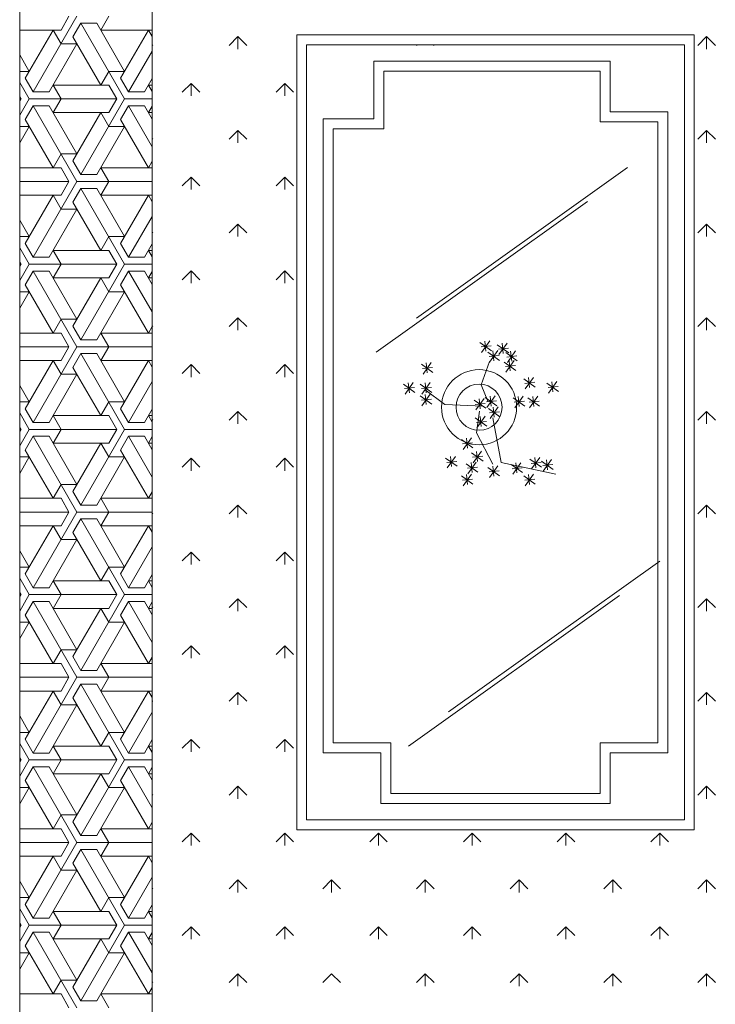
# Model space of a CAD drawing. Units: inches. Extents: x -1198 to -69, y -512 to 437.
# Tile 21 of 50: x -750 to -723, y 39 to 76. Entities that reach past the tile are written whole.
import ezdxf

# ---------------------------------------------------------------- set-up
doc = ezdxf.new("R2010")
doc.units = ezdxf.units.IN
doc.header["$MEASUREMENT"] = 0
doc.layers.add('A-FURN', color=60, linetype='Continuous', lineweight=18)

# ---------------------------------------------------------------- blocks, each defined once
blk = doc.blocks.new('A$C3B9F700E')
for p, q in [((1226.8, 1036.3, -685.7), (1240.1, 1049.6, -685.7)), ((1368.3, 1036.3, -685.7), (1381.5, 1049.6, -685.7)), ((1509.7, 1036.3, -685.7), (1522.9, 1049.6, -685.7)), ((1651.1, 1036.3, -685.7), (1664.4, 1049.6, -685.7)), ((1792.5, 1036.3, -685.7), (1805.8, 1049.6, -685.7)), ((1933.9, 1036.3, -685.7), (1947.2, 1049.6, -685.7)), ((2075.4, 1036.3, -685.7), (2088.6, 1049.6, -685.7)), ((2216.8, 1036.3, -685.7), (2230, 1049.6, -685.7)), ((2358.2, 1036.3, -685.7), (2371.5, 1049.6, -685.7)), ((2499.6, 1036.3, -685.7), (2512.9, 1049.6, -685.7)), ((2641.1, 1036.3, -685.7), (2654.3, 1049.6, -685.7)), ((1226.8, 1036.3, -685.7), (1240.1, 1023.1, -685.7)), ((1226.8, 1036.3, -685.7), (1245.6, 1036.3, -685.7)), ((1368.3, 1036.3, -685.7), (1381.5, 1023.1, -685.7)), ((1368.3, 1036.3, -685.7), (1387, 1036.3, -685.7)), ((1509.7, 1036.3, -685.7), (1522.9, 1023.1, -685.7)), ((1509.7, 1036.3, -685.7), (1528.4, 1036.3, -685.7)), ((1651.1, 1036.3, -685.7), (1664.4, 1023.1, -685.7)), ((1651.1, 1036.3, -685.7), (1669.9, 1036.3, -685.7)), ((1792.5, 1036.3, -685.7), (1805.8, 1023.1, -685.7)), ((1792.5, 1036.3, -685.7), (1811.3, 1036.3, -685.7)), ((1933.9, 1036.3, -685.7), (1947.2, 1023.1, -685.7)), ((1933.9, 1036.3, -685.7), (1952.7, 1036.3, -685.7)), ((2075.4, 1036.3, -685.7), (2088.6, 1023.1, -685.7)), ((2075.4, 1036.3, -685.7), (2094.1, 1036.3, -685.7)), ((2216.8, 1036.3, -685.7), (2230, 1023.1, -685.7)), ((2216.8, 1036.3, -685.7), (2235.5, 1036.3, -685.7)), ((2358.2, 1036.3, -685.7), (2371.5, 1023.1, -685.7)), ((2358.2, 1036.3, -685.7), (2377, 1036.3, -685.7)), ((2499.6, 1036.3, -685.7), (2512.9, 1023.1, -685.7)), ((2499.6, 1036.3, -685.7), (2518.4, 1036.3, -685.7)), ((2641.1, 1036.3, -685.7), (2654.3, 1023.1, -685.7)), ((2641.1, 1036.3, -685.7), (2659.8, 1036.3, -685.7)), ((1224, 417.9, -685.7), (1224, 1017.9, -685.7)), ((1224, 1017.9, -685.7), (2424, 1017.9, -685.7)), ((2424, 1017.9, -685.7), (2424, 417.9, -685.7)), ((1239, 432.9, -685.7), (1239, 1002.9, -685.7)), ((1239, 1002.9, -685.7), (2409, 1002.9, -685.7)), ((2409, 1002.9, -685.7), (2409, 432.9, -685.7)), ((1340.5, 977.9, -685.7), (2307.5, 977.9, -685.7)), ((1340.5, 890.9, -685.7), (1340.5, 977.9, -685.7)), ((2307.5, 977.9, -685.7), (2307.5, 890.9, -685.7)), ((2428.9, 965.6, -685.7), (2442.2, 978.9, -685.7)), ((2570.3, 965.6, -685.7), (2583.6, 978.9, -685.7)), ((1355.5, 962.9, -685.7), (2292.5, 962.9, -685.7)), ((1355.5, 875.9, -685.7), (1355.5, 962.9, -685.7)), ((2246, 647.2, -685.7), (2018.6, 965.9, -685.7)), ((2292.5, 962.9, -685.7), (2292.5, 875.9, -685.7)), ((2428.9, 965.6, -685.7), (2442.2, 952.3, -685.7)), ((2428.9, 965.6, -685.7), (2447.7, 965.6, -685.7)), ((2570.3, 965.6, -685.7), (2589.1, 965.6, -685.7)), ((2570.3, 965.6, -685.7), (2583.6, 952.3, -685.7)), ((1651.7, 598.7, -685.7), (1424.3, 917.3, -685.7)), ((2499.6, 894.9, -685.7), (2512.9, 908.1, -685.7)), ((2641.1, 894.9, -685.7), (2654.3, 908.1, -685.7)), ((2297.5, 586.5, -685.7), (2070.1, 905.2, -685.7)), ((2499.6, 894.9, -685.7), (2512.9, 881.6, -685.7)), ((2499.6, 894.9, -685.7), (2518.4, 894.9, -685.7)), ((2641.1, 894.9, -685.7), (2654.3, 881.6, -685.7)), ((2641.1, 894.9, -685.7), (2659.8, 894.9, -685.7)), ((1264, 534.4, -685.7), (1264, 890.9, -685.7)), ((1264, 890.9, -685.7), (1340.5, 890.9, -685.7)), ((2307.5, 890.9, -685.7), (2384, 890.9, -685.7)), ((2384, 890.9, -685.7), (2384, 544.9, -685.7)), ((1279, 549.4, -685.7), (1279, 875.9, -685.7)), ((1279, 875.9, -685.7), (1355.5, 875.9, -685.7)), ((2292.5, 875.9, -685.7), (2369, 875.9, -685.7)), ((2369, 875.9, -685.7), (2369, 559.9, -685.7)), ((1703.2, 538, -685.7), (1475.8, 856.6, -685.7)), ((2428.9, 824.2, -685.7), (2442.2, 837.4, -685.7)), ((2570.3, 824.2, -685.7), (2583.6, 837.4, -685.7)), ((2428.9, 824.2, -685.7), (2442.2, 810.9, -685.7)), ((2428.9, 824.2, -685.7), (2447.7, 824.2, -685.7)), ((2570.3, 824.2, -685.7), (2589.1, 824.2, -685.7)), ((2570.3, 824.2, -685.7), (2583.6, 810.9, -685.7)), ((1764.8, 797.9, -685.7), (1747.3, 810.4, -685.7)), ((1762.8, 804.4, -685.7), (1747.7, 802.8, -685.7)), ((1762.3, 812.9, -685.7), (1749.8, 795.4, -685.7)), ((1756.5, 797.3, -685.7), (1754.9, 812.4, -685.7)), ((1880, 805, -685.7), (1867.5, 787.5, -685.7)), ((1869.5, 726.5, -685.7), (1887, 808.9, -685.7)), ((1874.2, 789.3, -685.7), (1872.6, 804.4, -685.7)), ((1882.5, 790, -685.7), (1865, 802.5, -685.7)), ((1880.5, 796.5, -685.7), (1865.4, 794.9, -685.7)), ((1758.4, 762.9, -685.7), (1741, 775.4, -685.7)), ((1755.9, 777.9, -685.7), (1743.4, 760.4, -685.7)), ((1750.1, 762.2, -685.7), (1748.5, 777.4, -685.7)), ((1787.1, 769.3, -685.7), (1769.6, 781.8, -685.7)), ((1785.1, 775.8, -685.7), (1770, 774.2, -685.7)), ((1784.6, 784.3, -685.7), (1772.1, 766.8, -685.7)), ((1778.7, 768.6, -685.7), (1777.1, 783.7, -685.7)), ((1879.3, 772.4, -685.7), (1861.8, 784.9, -685.7)), ((1877.4, 779, -685.7), (1862.2, 777.4, -685.7)), ((1876.8, 787.4, -685.7), (1864.3, 769.9, -685.7)), ((1871, 771.8, -685.7), (1869.4, 786.9, -685.7)), ((1904.8, 762.9, -685.7), (1887.3, 775.4, -685.7)), ((1902.3, 777.9, -685.7), (1889.8, 760.4, -685.7)), ((1896.4, 762.2, -685.7), (1894.9, 777.4, -685.7)), ((1756.5, 769.4, -685.7), (1741.3, 767.8, -685.7)), ((1787.1, 747, -685.7), (1769.6, 759.5, -685.7)), ((1784.6, 762, -685.7), (1772.1, 744.5, -685.7)), ((1778.7, 746.3, -685.7), (1777.1, 761.4, -685.7)), ((1884.8, 758.8, -685.7), (1872.3, 741.3, -685.7)), ((1878.9, 743.1, -685.7), (1877.4, 758.3, -685.7)), ((1902.8, 769.4, -685.7), (1887.7, 767.8, -685.7)), ((2499.6, 753.5, -685.7), (2512.9, 766.7, -685.7)), ((2641.1, 753.5, -685.7), (2654.3, 766.7, -685.7)), ((1718.7, 735.8, -685.7), (1701.2, 748.3, -685.7)), ((1716.2, 750.8, -685.7), (1703.7, 733.3, -685.7)), ((1710.3, 735.2, -685.7), (1708.7, 750.3, -685.7)), ((1733, 733.4, -685.7), (1715.5, 745.9, -685.7)), ((1730.5, 748.4, -685.7), (1718, 730.9, -685.7)), ((1724.6, 732.8, -685.7), (1723.1, 747.9, -685.7)), ((1785.1, 753.5, -685.7), (1770, 751.9, -685.7)), ((1887.3, 743.8, -685.7), (1869.8, 756.3, -685.7)), ((1885.3, 750.3, -685.7), (1870.2, 748.7, -685.7)), ((2499.6, 753.5, -685.7), (2512.9, 740.2, -685.7)), ((2499.6, 753.5, -685.7), (2518.4, 753.5, -685.7)), ((2641.1, 753.5, -685.7), (2654.3, 740.2, -685.7)), ((2641.1, 753.5, -685.7), (2659.8, 753.5, -685.7)), ((1706.7, 723.1, -685.7), (1689.3, 735.6, -685.7)), ((1704.8, 729.6, -685.7), (1689.6, 728, -685.7)), ((1704.2, 738.1, -685.7), (1691.7, 720.6, -685.7)), ((1698.4, 722.4, -685.7), (1696.8, 737.6, -685.7)), ((1716.7, 742.3, -685.7), (1701.6, 740.7, -685.7)), ((1731, 740, -685.7), (1715.9, 738.4, -685.7)), ((1717.9, 708.8, -685.7), (1700.4, 721.3, -685.7)), ((1715.9, 715.3, -685.7), (1700.8, 713.7, -685.7)), ((1715.4, 723.8, -685.7), (1702.9, 706.3, -685.7)), ((1709.5, 708.1, -685.7), (1707.9, 723.2, -685.7)), ((1786.3, 704.8, -685.7), (1768.8, 717.3, -685.7)), ((1783.8, 719.8, -685.7), (1771.3, 702.3, -685.7)), ((1777.9, 704.1, -685.7), (1776.3, 719.3, -685.7)), ((1803, 709.6, -685.7), (1785.5, 722, -685.7)), ((1801, 716.1, -685.7), (1785.9, 714.5, -685.7)), ((1800.5, 724.5, -685.7), (1788, 707.1, -685.7)), ((1794.6, 708.9, -685.7), (1793, 724, -685.7)), ((1802.1, 714, -685.7), (1869.5, 726.5, -685.7)), ((1824.6, 689, -685.7), (1872, 714, -685.7)), ((1892, 708.8, -685.7), (1874.6, 721.3, -685.7)), ((1890.1, 715.3, -685.7), (1875, 713.7, -685.7)), ((1889.6, 723.8, -685.7), (1877.1, 706.3, -685.7)), ((1883.7, 708.1, -685.7), (1882.1, 723.2, -685.7)), ((1703.5, 696.8, -685.7), (1686.1, 709.3, -685.7)), ((1701.6, 703.3, -685.7), (1686.5, 701.7, -685.7)), ((1701, 711.8, -685.7), (1688.6, 694.3, -685.7)), ((1695.2, 696.2, -685.7), (1693.6, 711.3, -685.7)), ((1752.2, 696.5, -685.7), (1717.2, 709, -685.7)), ((1777.1, 706.5, -685.7), (1752.2, 696.5, -685.7)), ((1784.3, 711.3, -685.7), (1769.2, 709.7, -685.7)), ((1790.2, 688.1, -685.7), (1772.8, 700.6, -685.7)), ((1787.7, 703.1, -685.7), (1775.3, 685.6, -685.7)), ((1781.9, 687.4, -685.7), (1780.3, 702.5, -685.7)), ((1784.6, 699, -685.7), (1782.1, 641.6, -685.7)), ((1817.3, 689.7, -685.7), (1799.8, 702.1, -685.7)), ((1814.8, 704.6, -685.7), (1802.3, 687.2, -685.7)), ((1809, 689, -685.7), (1807.4, 704.1, -685.7)), ((1867.3, 699.1, -685.7), (1854.8, 681.6, -685.7)), ((1861.4, 683.4, -685.7), (1859.9, 698.6, -685.7)), ((1788.3, 694.6, -685.7), (1773.2, 693, -685.7)), ((1792.1, 694, -685.7), (1824.6, 689, -685.7)), ((1815.3, 696.2, -685.7), (1800.2, 694.6, -685.7)), ((1847.4, 683.9, -685.7), (1834.9, 666.5, -685.7)), ((1869.8, 684.1, -685.7), (1852.3, 696.6, -685.7)), ((1867.8, 690.6, -685.7), (1852.7, 689, -685.7)), ((1886.5, 676.1, -685.7), (1869, 688.6, -685.7)), ((1884, 691.1, -685.7), (1871.5, 673.6, -685.7)), ((1878.1, 675.5, -685.7), (1876.6, 690.6, -685.7)), ((1902.3, 683.9, -685.7), (1889.8, 666.5, -685.7)), ((2428.9, 682.8, -685.7), (2442.2, 696, -685.7)), ((2570.3, 682.8, -685.7), (2583.6, 696, -685.7)), ((1849.9, 669, -685.7), (1832.4, 681.5, -685.7)), ((1847.9, 675.5, -685.7), (1832.8, 673.9, -685.7)), ((1841.6, 668.3, -685.7), (1840, 683.4, -685.7)), ((1884.5, 682.6, -685.7), (1869.4, 681, -685.7)), ((1904.8, 669, -685.7), (1887.3, 681.5, -685.7)), ((1902.8, 675.5, -685.7), (1887.7, 673.9, -685.7)), ((1896.4, 668.3, -685.7), (1894.9, 683.4, -685.7)), ((2428.9, 682.8, -685.7), (2442.2, 669.5, -685.7)), ((2428.9, 682.8, -685.7), (2447.7, 682.8, -685.7)), ((2570.3, 682.8, -685.7), (2589.1, 682.8, -685.7)), ((2570.3, 682.8, -685.7), (2583.6, 669.5, -685.7)), ((1877.7, 645.1, -685.7), (1860.3, 657.6, -685.7)), ((1875.2, 660.1, -685.7), (1862.8, 642.6, -685.7)), ((1869.4, 644.4, -685.7), (1867.8, 659.5, -685.7)), ((1782.1, 641.6, -685.7), (1759.7, 611.6, -685.7)), ((1875.8, 651.6, -685.7), (1860.7, 650, -685.7)), ((1239, 624.2, -685.7), (1240.1, 625.3, -685.7)), ((2499.6, 612, -685.7), (2512.9, 625.3, -685.7)), ((2641.1, 612, -685.7), (2654.3, 625.3, -685.7)), ((1736.2, 608.5, -685.7), (1718.7, 621, -685.7)), ((1734.2, 615, -685.7), (1719.1, 613.4, -685.7)), ((1733.7, 623.4, -685.7), (1721.2, 606, -685.7)), ((1727.8, 607.8, -685.7), (1726.2, 622.9, -685.7)), ((1766.4, 606.9, -685.7), (1748.9, 619.4, -685.7)), ((1764.4, 613.4, -685.7), (1749.3, 611.8, -685.7)), ((1763.9, 621.9, -685.7), (1751.4, 604.4, -685.7)), ((1758, 606.2, -685.7), (1756.5, 621.3, -685.7)), ((1783.9, 606.9, -685.7), (1766.4, 619.4, -685.7)), ((1781.9, 613.4, -685.7), (1766.8, 611.8, -685.7)), ((1781.4, 621.9, -685.7), (1768.9, 604.4, -685.7)), ((1775.5, 606.2, -685.7), (1774, 621.3, -685.7)), ((2499.6, 612, -685.7), (2512.9, 598.8, -685.7)), ((2499.6, 612, -685.7), (2518.4, 612, -685.7)), ((2641.1, 612, -685.7), (2654.3, 598.8, -685.7)), ((2641.1, 612, -685.7), (2659.8, 612, -685.7)), ((1239, 599.9, -685.7), (1240.1, 598.8, -685.7)), ((1763.9, 596.4, -685.7), (1751.4, 578.9, -685.7)), ((1758, 580.7, -685.7), (1756.5, 595.9, -685.7)), ((1766.4, 581.4, -685.7), (1748.9, 593.9, -685.7)), ((1764.4, 587.9, -685.7), (1749.3, 586.3, -685.7)), ((2292.5, 559.9, -685.7), (2292.5, 472.9, -685.7)), ((2369, 559.9, -685.7), (2292.5, 559.9, -685.7)), ((2428.9, 541.3, -685.7), (2442.2, 554.6, -685.7)), ((2570.3, 541.3, -685.7), (2583.6, 554.6, -685.7)), ((1366, 549.4, -685.7), (1279, 549.4, -685.7)), ((1366, 472.9, -685.7), (1366, 549.4, -685.7)), ((2307.5, 544.9, -685.7), (2307.5, 457.9, -685.7)), ((2384, 544.9, -685.7), (2307.5, 544.9, -685.7)), ((2428.9, 541.3, -685.7), (2442.2, 528.1, -685.7)), ((2428.9, 541.3, -685.7), (2447.7, 541.3, -685.7)), ((2570.3, 541.3, -685.7), (2589.1, 541.3, -685.7)), ((2570.3, 541.3, -685.7), (2583.6, 528.1, -685.7)), ((1351, 534.4, -685.7), (1264, 534.4, -685.7)), ((1351, 457.9, -685.7), (1351, 534.4, -685.7)), ((2499.6, 470.6, -685.7), (2512.9, 483.9, -685.7)), ((2641.1, 470.6, -685.7), (2654.3, 483.9, -685.7)), ((2292.5, 472.9, -685.7), (1366, 472.9, -685.7)), ((2499.6, 470.6, -685.7), (2518.4, 470.6, -685.7)), ((2499.6, 470.6, -685.7), (2512.9, 457.4, -685.7)), ((2641.1, 470.6, -685.7), (2654.3, 457.4, -685.7)), ((2307.5, 457.9, -685.7), (1351, 457.9, -685.7)), ((2409, 432.9, -685.7), (1239, 432.9, -685.7)), ((2424, 417.9, -685.7), (1224, 417.9, -685.7)), ((1297.5, 399.9, -685.7), (1310.8, 413.2, -685.7)), ((1439, 399.9, -685.7), (1452.2, 413.2, -685.7)), ((1580.4, 399.9, -685.7), (1593.6, 413.2, -685.7)), ((1721.8, 399.9, -685.7), (1735.1, 413.2, -685.7)), ((1863.2, 399.9, -685.7), (1876.5, 413.2, -685.7)), ((2004.7, 399.9, -685.7), (2017.9, 413.2, -685.7)), ((2146.1, 399.9, -685.7), (2159.3, 413.2, -685.7)), ((2287.5, 399.9, -685.7), (2300.8, 413.2, -685.7)), ((2428.9, 399.9, -685.7), (2442.2, 413.2, -685.7)), ((2570.3, 399.9, -685.7), (2583.6, 413.2, -685.7)), ((1297.5, 399.9, -685.7), (1316.3, 399.9, -685.7)), ((1297.5, 399.9, -685.7), (1310.8, 386.7, -685.7)), ((1439, 399.9, -685.7), (1457.7, 399.9, -685.7)), ((1439, 399.9, -685.7), (1452.2, 386.7, -685.7)), ((1580.4, 399.9, -685.7), (1599.1, 399.9, -685.7)), ((1580.4, 399.9, -685.7), (1593.6, 386.7, -685.7)), ((1721.8, 399.9, -685.7), (1740.6, 399.9, -685.7)), ((1721.8, 399.9, -685.7), (1735.1, 386.7, -685.7)), ((1863.2, 399.9, -685.7), (1882, 399.9, -685.7)), ((1863.2, 399.9, -685.7), (1876.5, 386.7, -685.7)), ((2004.7, 399.9, -685.7), (2023.4, 399.9, -685.7)), ((2004.7, 399.9, -685.7), (2017.9, 386.7, -685.7)), ((2146.1, 399.9, -685.7), (2164.8, 399.9, -685.7)), ((2146.1, 399.9, -685.7), (2159.3, 386.7, -685.7)), ((2287.5, 399.9, -685.7), (2306.2, 399.9, -685.7)), ((2287.5, 399.9, -685.7), (2300.8, 386.7, -685.7)), ((2428.9, 399.9, -685.7), (2447.7, 399.9, -685.7)), ((2428.9, 399.9, -685.7), (2442.2, 386.7, -685.7)), ((2570.3, 399.9, -685.7), (2589.1, 399.9, -685.7)), ((2570.3, 399.9, -685.7), (2583.6, 386.7, -685.7)), ((1226.8, 329.2, -685.7), (1240.1, 342.5, -685.7)), ((1368.3, 329.2, -685.7), (1381.5, 342.5, -685.7)), ((1509.7, 329.2, -685.7), (1522.9, 342.5, -685.7)), ((1651.1, 329.2, -685.7), (1664.4, 342.5, -685.7)), ((1792.5, 329.2, -685.7), (1805.8, 342.5, -685.7)), ((1933.9, 329.2, -685.7), (1947.2, 342.5, -685.7)), ((2075.4, 329.2, -685.7), (2088.6, 342.5, -685.7)), ((2216.8, 329.2, -685.7), (2230, 342.5, -685.7)), ((2358.2, 329.2, -685.7), (2371.5, 342.5, -685.7)), ((2499.6, 329.2, -685.7), (2512.9, 342.5, -685.7)), ((2641.1, 329.2, -685.7), (2654.3, 342.5, -685.7)), ((1226.8, 329.2, -685.7), (1240.1, 315.9, -685.7)), ((1226.8, 329.2, -685.7), (1245.6, 329.2, -685.7)), ((1368.3, 329.2, -685.7), (1381.5, 315.9, -685.7)), ((1368.3, 329.2, -685.7), (1387, 329.2, -685.7)), ((1509.7, 329.2, -685.7), (1522.9, 315.9, -685.7)), ((1509.7, 329.2, -685.7), (1528.4, 329.2, -685.7)), ((1651.1, 329.2, -685.7), (1664.4, 315.9, -685.7)), ((1651.1, 329.2, -685.7), (1669.9, 329.2, -685.7)), ((1792.5, 329.2, -685.7), (1805.8, 315.9, -685.7)), ((1792.5, 329.2, -685.7), (1811.3, 329.2, -685.7)), ((1933.9, 329.2, -685.7), (1947.2, 315.9, -685.7)), ((1933.9, 329.2, -685.7), (1952.7, 329.2, -685.7)), ((2075.4, 329.2, -685.7), (2088.6, 315.9, -685.7)), ((2075.4, 329.2, -685.7), (2094.1, 329.2, -685.7)), ((2216.8, 329.2, -685.7), (2230, 315.9, -685.7)), ((2216.8, 329.2, -685.7), (2235.5, 329.2, -685.7)), ((2358.2, 329.2, -685.7), (2371.5, 315.9, -685.7)), ((2358.2, 329.2, -685.7), (2377, 329.2, -685.7)), ((2499.6, 329.2, -685.7), (2512.9, 315.9, -685.7)), ((2499.6, 329.2, -685.7), (2518.4, 329.2, -685.7)), ((2641.1, 329.2, -685.7), (2654.3, 315.9, -685.7)), ((2641.1, 329.2, -685.7), (2659.8, 329.2, -685.7)), ((1297.5, 258.5, -685.7), (1310.8, 271.8, -685.7)), ((1439, 258.5, -685.7), (1452.2, 271.8, -685.7)), ((1580.4, 258.5, -685.7), (1593.6, 271.8, -685.7)), ((1721.8, 258.5, -685.7), (1735.1, 271.8, -685.7)), ((1863.2, 258.5, -685.7), (1876.5, 271.8, -685.7)), ((2004.7, 258.5, -685.7), (2017.9, 271.8, -685.7)), ((2146.1, 258.5, -685.7), (2159.3, 271.8, -685.7)), ((2287.5, 258.5, -685.7), (2300.8, 271.8, -685.7)), ((2428.9, 258.5, -685.7), (2442.2, 271.8, -685.7)), ((2570.3, 258.5, -685.7), (2583.6, 271.8, -685.7)), ((1297.5, 258.5, -685.7), (1310.8, 245.2, -685.7)), ((1297.5, 258.5, -685.7), (1316.3, 258.5, -685.7)), ((1439, 258.5, -685.7), (1452.2, 245.2, -685.7)), ((1439, 258.5, -685.7), (1457.7, 258.5, -685.7)), ((1580.4, 258.5, -685.7), (1593.6, 245.2, -685.7)), ((1580.4, 258.5, -685.7), (1599.1, 258.5, -685.7)), ((1721.8, 258.5, -685.7), (1735.1, 245.2, -685.7)), ((1721.8, 258.5, -685.7), (1740.6, 258.5, -685.7)), ((1863.2, 258.5, -685.7), (1876.5, 245.2, -685.7)), ((1863.2, 258.5, -685.7), (1882, 258.5, -685.7)), ((2004.7, 258.5, -685.7), (2017.9, 245.2, -685.7)), ((2004.7, 258.5, -685.7), (2023.4, 258.5, -685.7)), ((2146.1, 258.5, -685.7), (2159.3, 245.2, -685.7)), ((2146.1, 258.5, -685.7), (2164.8, 258.5, -685.7)), ((2287.5, 258.5, -685.7), (2300.8, 245.2, -685.7)), ((2287.5, 258.5, -685.7), (2306.2, 258.5, -685.7)), ((2428.9, 258.5, -685.7), (2442.2, 245.2, -685.7)), ((2428.9, 258.5, -685.7), (2447.7, 258.5, -685.7)), ((2570.3, 258.5, -685.7), (2589.1, 258.5, -685.7)), ((2570.3, 258.5, -685.7), (2583.6, 245.2, -685.7)), ((3062.1, 200, -685.7), (601.4, 200, -685.7)), ((3062.1, 200, -685.7), (601.4, 200, -685.7)), ((1216.8, 200, -685.7), (1216.8, 122.3, -685.7)), ((1226.6, 200, -685.7), (1216.8, 194.3, -685.7)), ((1289.6, 152.3, -685.7), (1216.8, 194.3, -685.7)), ((1239.1, 200, -685.7), (1240.1, 201, -685.7)), ((1248.5, 200, -685.7), (1310.3, 164.3, -685.7)), ((1310.3, 188.3, -685.7), (1290.1, 200, -685.7)), ((1299.9, 200, -685.7), (1299.9, 194.3, -685.7)), ((1309.8, 200, -685.7), (1299.9, 194.3, -685.7)), ((1320.7, 158.3, -685.7), (1320.7, 200, -685.7)), ((1331.1, 188.3, -685.7), (1351.3, 200, -685.7)), ((1392.9, 200, -685.7), (1331.1, 164.3, -685.7)), ((1331.7, 200, -685.7), (1341.5, 194.3, -685.7)), ((1341.5, 200, -685.7), (1341.5, 194.3, -685.7)), ((1351.9, 152.3, -685.7), (1424.7, 194.3, -685.7)), ((1380.5, 200, -685.7), (1381.5, 201, -685.7)), ((1414.8, 200, -685.7), (1424.7, 194.3, -685.7)), ((1424.7, 200, -685.7), (1424.7, 122.3, -685.7)), ((1445.4, 86.3, -685.7), (1445.4, 200, -685.7)), ((1466.2, 200, -685.7), (1466.2, 122.3, -685.7)), ((1476.1, 200, -685.7), (1466.2, 194.3, -685.7)), ((1539, 152.3, -685.7), (1466.2, 194.3, -685.7)), ((1498, 200, -685.7), (1559.8, 164.3, -685.7)), ((1521.9, 200, -685.7), (1522.9, 201, -685.7)), ((1559.8, 188.3, -685.7), (1539.5, 200, -685.7)), ((1549.4, 200, -685.7), (1549.4, 194.3, -685.7)), ((1559.2, 200, -685.7), (1549.4, 194.3, -685.7)), ((1570.1, 158.3, -685.7), (1570.1, 200, -685.7)), ((1580.5, 188.3, -685.7), (1600.8, 200, -685.7)), ((1642.3, 200, -685.7), (1580.5, 164.3, -685.7)), ((1581.1, 200, -685.7), (1590.9, 194.3, -685.7)), ((1590.9, 200, -685.7), (1590.9, 194.3, -685.7)), ((1601.3, 152.3, -685.7), (1674.1, 194.3, -685.7)), ((1663.3, 200, -685.7), (1664.4, 201, -685.7)), ((1664.2, 200, -685.7), (1674.1, 194.3, -685.7)), ((1674.1, 200, -685.7), (1674.1, 122.3, -685.7)), ((1694.9, 86.3, -685.7), (1694.9, 200, -685.7)), ((1715.6, 200, -685.7), (1715.6, 122.3, -685.7)), ((1725.5, 200, -685.7), (1715.6, 194.3, -685.7)), ((1788.4, 152.3, -685.7), (1715.6, 194.3, -685.7)), ((1747.4, 200, -685.7), (1809.2, 164.3, -685.7)), ((1809.2, 188.3, -685.7), (1788.9, 200, -685.7)), ((1798.8, 200, -685.7), (1798.8, 194.3, -685.7)), ((1808.6, 200, -685.7), (1798.8, 194.3, -685.7)), ((1804.7, 200, -685.7), (1805.8, 201, -685.7)), ((1819.6, 158.3, -685.7), (1819.6, 200, -685.7)), ((1830, 188.3, -685.7), (1850.2, 200, -685.7)), ((1891.7, 200, -685.7), (1830, 164.3, -685.7)), ((1830.5, 200, -685.7), (1840.3, 194.3, -685.7)), ((1840.3, 200, -685.7), (1840.3, 194.3, -685.7)), ((1850.7, 152.3, -685.7), (1923.5, 194.3, -685.7)), ((1913.6, 200, -685.7), (1923.5, 194.3, -685.7)), ((1923.5, 200, -685.7), (1923.5, 122.3, -685.7)), ((1944.3, 86.3, -685.7), (1944.3, 200, -685.7)), ((1946.2, 200, -685.7), (1947.2, 201, -685.7)), ((1965.1, 200, -685.7), (1965.1, 122.3, -685.7)), ((1974.9, 200, -685.7), (1965.1, 194.3, -685.7)), ((2037.8, 152.3, -685.7), (1965.1, 194.3, -685.7)), ((1996.8, 200, -685.7), (2058.6, 164.3, -685.7)), ((2058.6, 188.3, -685.7), (2038.4, 200, -685.7)), ((2048.2, 200, -685.7), (2048.2, 194.3, -685.7)), ((2058, 200, -685.7), (2048.2, 194.3, -685.7)), ((2069, 158.3, -685.7), (2069, 200, -685.7)), ((2079.4, 188.3, -685.7), (2099.6, 200, -685.7)), ((2141.2, 200, -685.7), (2079.4, 164.3, -685.7)), ((2079.9, 200, -685.7), (2089.8, 194.3, -685.7)), ((2087.6, 200, -685.7), (2088.6, 201, -685.7)), ((2089.8, 200, -685.7), (2089.8, 194.3, -685.7)), ((2100.2, 152.3, -685.7), (2172.9, 194.3, -685.7)), ((2163.1, 200, -685.7), (2172.9, 194.3, -685.7)), ((2172.9, 200, -685.7), (2172.9, 122.3, -685.7)), ((2193.7, 86.3, -685.7), (2193.7, 200, -685.7)), ((2214.5, 200, -685.7), (2214.5, 122.3, -685.7)), ((2224.3, 200, -685.7), (2214.5, 194.3, -685.7)), ((2287.2, 152.3, -685.7), (2214.5, 194.3, -685.7)), ((2229, 200, -685.7), (2230, 201, -685.7)), ((2246.2, 200, -685.7), (2308, 164.3, -685.7)), ((2308, 188.3, -685.7), (2287.8, 200, -685.7)), ((2297.6, 200, -685.7), (2297.6, 194.3, -685.7)), ((2307.4, 200, -685.7), (2297.6, 194.3, -685.7)), ((2318.4, 158.3, -685.7), (2318.4, 200, -685.7)), ((2328.8, 188.3, -685.7), (2349, 200, -685.7)), ((2390.6, 200, -685.7), (2328.8, 164.3, -685.7)), ((2329.3, 200, -685.7), (2339.2, 194.3, -685.7)), ((2339.2, 200, -685.7), (2339.2, 194.3, -685.7)), ((2349.6, 152.3, -685.7), (2422.3, 194.3, -685.7)), ((2370.4, 200, -685.7), (2371.5, 201, -685.7)), ((2412.5, 200, -685.7), (2422.3, 194.3, -685.7)), ((2422.3, 200, -685.7), (2422.3, 122.3, -685.7)), ((2443.1, 86.3, -685.7), (2443.1, 200, -685.7)), ((2463.9, 200, -685.7), (2463.9, 122.3, -685.7)), ((2473.7, 200, -685.7), (2463.9, 194.3, -685.7)), ((2536.6, 152.3, -685.7), (2463.9, 194.3, -685.7)), ((2495.6, 200, -685.7), (2557.4, 164.3, -685.7)), ((2511.8, 200, -685.7), (2512.9, 201, -685.7)), ((2557.4, 188.3, -685.7), (2537.2, 200, -685.7)), ((2547, 200, -685.7), (2547, 194.3, -685.7)), ((2556.9, 200, -685.7), (2547, 194.3, -685.7)), ((2567.8, 158.3, -685.7), (2567.8, 200, -685.7)), ((2578.2, 188.3, -685.7), (2598.4, 200, -685.7)), ((2640, 200, -685.7), (2578.2, 164.3, -685.7)), ((2578.8, 200, -685.7), (2588.6, 194.3, -685.7)), ((2588.6, 200, -685.7), (2588.6, 194.3, -685.7)), ((2599, 152.3, -685.7), (2671.7, 194.3, -685.7)), ((2653.3, 200, -685.7), (2654.3, 201, -685.7)), ((2661.9, 200, -685.7), (2671.7, 194.3, -685.7)), ((2671.7, 200, -685.7), (2671.7, 122.3, -685.7)), ((1310.3, 164.3, -685.7), (1310.3, 188.3, -685.7)), ((1331.1, 164.3, -685.7), (1331.1, 188.3, -685.7)), ((1559.8, 164.3, -685.7), (1559.8, 188.3, -685.7)), ((1580.5, 164.3, -685.7), (1580.5, 188.3, -685.7)), ((1809.2, 164.3, -685.7), (1809.2, 188.3, -685.7)), ((1830, 164.3, -685.7), (1830, 188.3, -685.7)), ((2058.6, 164.3, -685.7), (2058.6, 188.3, -685.7)), ((2079.4, 164.3, -685.7), (2079.4, 188.3, -685.7)), ((2308, 164.3, -685.7), (2308, 188.3, -685.7)), ((2328.8, 164.3, -685.7), (2328.8, 188.3, -685.7)), ((2557.4, 164.3, -685.7), (2557.4, 188.3, -685.7)), ((2578.2, 164.3, -685.7), (2578.2, 188.3, -685.7)), ((1310.3, 164.3, -685.7), (1289.6, 152.3, -685.7)), ((1331.1, 164.3, -685.7), (1351.9, 152.3, -685.7)), ((1559.8, 164.3, -685.7), (1539, 152.3, -685.7)), ((1580.5, 164.3, -685.7), (1601.3, 152.3, -685.7)), ((1809.2, 164.3, -685.7), (1788.4, 152.3, -685.7)), ((1830, 164.3, -685.7), (1850.7, 152.3, -685.7)), ((2058.6, 164.3, -685.7), (2037.8, 152.3, -685.7)), ((2079.4, 164.3, -685.7), (2100.2, 152.3, -685.7)), ((2308, 164.3, -685.7), (2287.2, 152.3, -685.7)), ((2328.8, 164.3, -685.7), (2349.6, 152.3, -685.7)), ((2557.4, 164.3, -685.7), (2536.6, 152.3, -685.7)), ((2578.2, 164.3, -685.7), (2599, 152.3, -685.7)), ((1206.4, 116.3, -685.7), (1279.2, 158.3, -685.7)), ((1320.7, 158.3, -685.7), (1206.4, 92.3, -685.7)), ((1279.2, 134.3, -685.7), (1279.2, 158.3, -685.7)), ((1320.7, 158.3, -685.7), (1435, 92.3, -685.7)), ((1435, 116.3, -685.7), (1362.3, 158.3, -685.7)), ((1362.3, 134.3, -685.7), (1362.3, 158.3, -685.7)), ((1455.8, 116.3, -685.7), (1528.6, 158.3, -685.7)), ((1570.1, 158.3, -685.7), (1455.8, 92.3, -685.7)), ((1528.6, 134.3, -685.7), (1528.6, 158.3, -685.7)), ((1570.1, 158.3, -685.7), (1684.5, 92.3, -685.7)), ((1684.5, 116.3, -685.7), (1611.7, 158.3, -685.7)), ((1611.7, 134.3, -685.7), (1611.7, 158.3, -685.7)), ((1705.2, 116.3, -685.7), (1778, 158.3, -685.7)), ((1819.6, 158.3, -685.7), (1705.2, 92.3, -685.7)), ((1778, 134.3, -685.7), (1778, 158.3, -685.7)), ((1819.6, 158.3, -685.7), (1933.9, 92.3, -685.7)), ((1933.9, 116.3, -685.7), (1861.1, 158.3, -685.7)), ((1861.1, 134.3, -685.7), (1861.1, 158.3, -685.7)), ((1954.7, 116.3, -685.7), (2027.4, 158.3, -685.7)), ((2069, 158.3, -685.7), (1954.7, 92.3, -685.7)), ((2027.4, 134.3, -685.7), (2027.4, 158.3, -685.7)), ((2069, 158.3, -685.7), (2183.3, 92.3, -685.7)), ((2183.3, 116.3, -685.7), (2110.5, 158.3, -685.7)), ((2110.5, 134.3, -685.7), (2110.5, 158.3, -685.7)), ((2204.1, 116.3, -685.7), (2276.8, 158.3, -685.7)), ((2318.4, 158.3, -685.7), (2204.1, 92.3, -685.7)), ((2276.8, 134.3, -685.7), (2276.8, 158.3, -685.7)), ((2318.4, 158.3, -685.7), (2432.7, 92.3, -685.7)), ((2432.7, 116.3, -685.7), (2360, 158.3, -685.7)), ((2360, 134.3, -685.7), (2360, 158.3, -685.7)), ((2453.5, 116.3, -685.7), (2526.2, 158.3, -685.7)), ((2567.8, 158.3, -685.7), (2453.5, 92.3, -685.7)), ((2526.2, 134.3, -685.7), (2526.2, 158.3, -685.7)), ((2567.8, 158.3, -685.7), (2682.1, 92.3, -685.7)), ((2682.1, 116.3, -685.7), (2609.4, 158.3, -685.7)), ((2609.4, 134.3, -685.7), (2609.4, 158.3, -685.7)), ((1196, 134.3, -685.7), (1216.8, 122.3, -685.7)), ((1279.2, 134.3, -685.7), (1299.9, 122.3, -685.7)), ((1320.7, 146.3, -685.7), (1299.9, 134.3, -685.7)), ((1299.9, 134.3, -685.7), (1299.9, 50.3, -685.7)), ((1320.7, 146.3, -685.7), (1341.5, 134.3, -685.7)), ((1320.7, 14.3, -685.7), (1320.7, 146.3, -685.7)), ((1341.5, 134.3, -685.7), (1341.5, 50.3, -685.7)), ((1362.3, 134.3, -685.7), (1341.5, 122.3, -685.7)), ((1445.4, 134.3, -685.7), (1424.7, 122.3, -685.7)), ((1445.4, 134.3, -685.7), (1466.2, 122.3, -685.7)), ((1528.6, 134.3, -685.7), (1549.4, 122.3, -685.7)), ((1570.1, 146.3, -685.7), (1549.4, 134.3, -685.7)), ((1549.4, 134.3, -685.7), (1549.4, 50.3, -685.7)), ((1570.1, 146.3, -685.7), (1590.9, 134.3, -685.7)), ((1570.1, 14.3, -685.7), (1570.1, 146.3, -685.7)), ((1590.9, 134.3, -685.7), (1590.9, 50.3, -685.7)), ((1611.7, 134.3, -685.7), (1590.9, 122.3, -685.7)), ((1694.9, 134.3, -685.7), (1674.1, 122.3, -685.7)), ((1694.9, 134.3, -685.7), (1715.6, 122.3, -685.7)), ((1778, 134.3, -685.7), (1798.8, 122.3, -685.7)), ((1819.6, 146.3, -685.7), (1798.8, 134.3, -685.7)), ((1798.8, 134.3, -685.7), (1798.8, 50.3, -685.7)), ((1819.6, 146.3, -685.7), (1840.3, 134.3, -685.7)), ((1819.6, 14.3, -685.7), (1819.6, 146.3, -685.7)), ((1840.3, 134.3, -685.7), (1840.3, 50.3, -685.7)), ((1861.1, 134.3, -685.7), (1840.3, 122.3, -685.7)), ((1944.3, 134.3, -685.7), (1923.5, 122.3, -685.7)), ((1944.3, 134.3, -685.7), (1965.1, 122.3, -685.7)), ((2027.4, 134.3, -685.7), (2048.2, 122.3, -685.7)), ((2069, 146.3, -685.7), (2048.2, 134.3, -685.7)), ((2048.2, 134.3, -685.7), (2048.2, 50.3, -685.7)), ((2069, 146.3, -685.7), (2089.8, 134.3, -685.7)), ((2069, 14.3, -685.7), (2069, 146.3, -685.7)), ((2089.8, 134.3, -685.7), (2089.8, 50.3, -685.7)), ((2110.5, 134.3, -685.7), (2089.8, 122.3, -685.7)), ((2193.7, 134.3, -685.7), (2172.9, 122.3, -685.7)), ((2193.7, 134.3, -685.7), (2214.5, 122.3, -685.7)), ((2276.8, 134.3, -685.7), (2297.6, 122.3, -685.7)), ((2318.4, 146.3, -685.7), (2297.6, 134.3, -685.7)), ((2297.6, 134.3, -685.7), (2297.6, 50.3, -685.7)), ((2318.4, 146.3, -685.7), (2339.2, 134.3, -685.7)), ((2318.4, 14.3, -685.7), (2318.4, 146.3, -685.7)), ((2339.2, 134.3, -685.7), (2339.2, 50.3, -685.7)), ((2360, 134.3, -685.7), (2339.2, 122.3, -685.7)), ((2443.1, 134.3, -685.7), (2422.3, 122.3, -685.7)), ((2443.1, 134.3, -685.7), (2463.9, 122.3, -685.7)), ((2526.2, 134.3, -685.7), (2547, 122.3, -685.7)), ((2567.8, 146.3, -685.7), (2547, 134.3, -685.7)), ((2547, 134.3, -685.7), (2547, 50.3, -685.7)), ((2567.8, 146.3, -685.7), (2588.6, 134.3, -685.7)), ((2567.8, 14.3, -685.7), (2567.8, 146.3, -685.7)), ((2588.6, 134.3, -685.7), (2588.6, 50.3, -685.7)), ((2609.4, 134.3, -685.7), (2588.6, 122.3, -685.7)), ((2692.5, 134.3, -685.7), (2671.7, 122.3, -685.7)), ((1227.2, 80.3, -685.7), (1299.9, 122.3, -685.7)), ((1414.3, 80.3, -685.7), (1341.5, 122.3, -685.7)), ((1476.6, 80.3, -685.7), (1549.4, 122.3, -685.7)), ((1663.7, 80.3, -685.7), (1590.9, 122.3, -685.7)), ((1726, 80.3, -685.7), (1798.8, 122.3, -685.7)), ((1913.1, 80.3, -685.7), (1840.3, 122.3, -685.7)), ((1975.4, 80.3, -685.7), (2048.2, 122.3, -685.7)), ((2162.5, 80.3, -685.7), (2089.8, 122.3, -685.7)), ((2224.9, 80.3, -685.7), (2297.6, 122.3, -685.7)), ((2411.9, 80.3, -685.7), (2339.2, 122.3, -685.7)), ((2474.3, 80.3, -685.7), (2547, 122.3, -685.7)), ((2661.3, 80.3, -685.7), (2588.6, 122.3, -685.7)), ((1206.4, 92.3, -685.7), (1206.4, 116.3, -685.7)), ((1435, 92.3, -685.7), (1435, 116.3, -685.7)), ((1455.8, 92.3, -685.7), (1455.8, 116.3, -685.7)), ((1684.5, 92.3, -685.7), (1684.5, 116.3, -685.7)), ((1705.2, 92.3, -685.7), (1705.2, 116.3, -685.7)), ((1933.9, 92.3, -685.7), (1933.9, 116.3, -685.7)), ((1954.7, 92.3, -685.7), (1954.7, 116.3, -685.7)), ((2183.3, 92.3, -685.7), (2183.3, 116.3, -685.7)), ((2204.1, 92.3, -685.7), (2204.1, 116.3, -685.7)), ((2432.7, 92.3, -685.7), (2432.7, 116.3, -685.7)), ((2453.5, 92.3, -685.7), (2453.5, 116.3, -685.7)), ((2682.1, 92.3, -685.7), (2682.1, 116.3, -685.7)), ((1206.4, 92.3, -685.7), (1227.2, 80.3, -685.7)), ((1435, 92.3, -685.7), (1414.3, 80.3, -685.7)), ((1455.8, 92.3, -685.7), (1476.6, 80.3, -685.7)), ((1684.5, 92.3, -685.7), (1663.7, 80.3, -685.7)), ((1705.2, 92.3, -685.7), (1726, 80.3, -685.7)), ((1933.9, 92.3, -685.7), (1913.1, 80.3, -685.7)), ((1954.7, 92.3, -685.7), (1975.4, 80.3, -685.7)), ((2183.3, 92.3, -685.7), (2162.5, 80.3, -685.7)), ((2204.1, 92.3, -685.7), (2224.9, 80.3, -685.7)), ((2432.7, 92.3, -685.7), (2411.9, 80.3, -685.7)), ((2453.5, 92.3, -685.7), (2474.3, 80.3, -685.7)), ((2682.1, 92.3, -685.7), (2661.3, 80.3, -685.7)), ((1196, 86.3, -685.7), (1310.3, 20.3, -685.7)), ((1196, 74.3, -685.7), (1216.8, 62.3, -685.7)), ((1310.3, 44.3, -685.7), (1237.6, 86.3, -685.7)), ((1237.6, 62.3, -685.7), (1237.6, 86.3, -685.7)), ((1331.1, 44.3, -685.7), (1403.9, 86.3, -685.7)), ((1445.4, 86.3, -685.7), (1331.1, 20.3, -685.7)), ((1403.9, 62.3, -685.7), (1403.9, 86.3, -685.7)), ((1445.4, 74.3, -685.7), (1424.7, 62.3, -685.7)), ((1445.4, 86.3, -685.7), (1559.8, 20.3, -685.7)), ((1445.4, 74.3, -685.7), (1466.2, 62.3, -685.7)), ((1445.4, 0, -685.7), (1445.4, 74.3, -685.7)), ((1487, 62.3, -685.7), (1487, 86.3, -685.7)), ((1559.8, 44.3, -685.7), (1487, 86.3, -685.7)), ((1580.5, 44.3, -685.7), (1653.3, 86.3, -685.7)), ((1694.9, 86.3, -685.7), (1580.5, 20.3, -685.7)), ((1653.3, 62.3, -685.7), (1653.3, 86.3, -685.7)), ((1694.9, 74.3, -685.7), (1674.1, 62.3, -685.7)), ((1694.9, 86.3, -685.7), (1809.2, 20.3, -685.7)), ((1694.9, 74.3, -685.7), (1715.6, 62.3, -685.7)), ((1694.9, 0, -685.7), (1694.9, 74.3, -685.7)), ((1809.2, 44.3, -685.7), (1736.4, 86.3, -685.7)), ((1736.4, 62.3, -685.7), (1736.4, 86.3, -685.7)), ((1830, 44.3, -685.7), (1902.7, 86.3, -685.7)), ((1944.3, 86.3, -685.7), (1830, 20.3, -685.7)), ((1902.7, 62.3, -685.7), (1902.7, 86.3, -685.7)), ((1944.3, 74.3, -685.7), (1923.5, 62.3, -685.7)), ((1944.3, 86.3, -685.7), (2058.6, 20.3, -685.7)), ((1944.3, 74.3, -685.7), (1965.1, 62.3, -685.7)), ((1944.3, 0, -685.7), (1944.3, 74.3, -685.7)), ((1985.8, 62.3, -685.7), (1985.8, 86.3, -685.7)), ((2058.6, 44.3, -685.7), (1985.8, 86.3, -685.7)), ((2079.4, 44.3, -685.7), (2152.1, 86.3, -685.7)), ((2193.7, 86.3, -685.7), (2079.4, 20.3, -685.7)), ((2152.1, 62.3, -685.7), (2152.1, 86.3, -685.7)), ((2193.7, 74.3, -685.7), (2172.9, 62.3, -685.7)), ((2193.7, 86.3, -685.7), (2308, 20.3, -685.7)), ((2193.7, 74.3, -685.7), (2214.5, 62.3, -685.7)), ((2193.7, 0, -685.7), (2193.7, 74.3, -685.7)), ((2308, 44.3, -685.7), (2235.3, 86.3, -685.7)), ((2235.3, 62.3, -685.7), (2235.3, 86.3, -685.7)), ((2328.8, 44.3, -685.7), (2401.5, 86.3, -685.7)), ((2443.1, 86.3, -685.7), (2328.8, 20.3, -685.7)), ((2401.5, 62.3, -685.7), (2401.5, 86.3, -685.7)), ((2443.1, 74.3, -685.7), (2422.3, 62.3, -685.7)), ((2443.1, 86.3, -685.7), (2557.4, 20.3, -685.7)), ((2443.1, 74.3, -685.7), (2463.9, 62.3, -685.7)), ((2443.1, 0, -685.7), (2443.1, 74.3, -685.7)), ((2484.7, 62.3, -685.7), (2484.7, 86.3, -685.7)), ((2557.4, 44.3, -685.7), (2484.7, 86.3, -685.7)), ((2578.2, 44.3, -685.7), (2650.9, 86.3, -685.7)), ((2692.5, 86.3, -685.7), (2578.2, 20.3, -685.7)), ((2650.9, 62.3, -685.7), (2650.9, 86.3, -685.7)), ((2692.5, 74.3, -685.7), (2671.7, 62.3, -685.7)), ((1216.8, 62.3, -685.7), (1216.8, 0, -685.7)), ((1237.6, 62.3, -685.7), (1216.8, 50.3, -685.7)), ((1320.7, 62.3, -685.7), (1299.9, 50.3, -685.7)), ((1320.7, 62.3, -685.7), (1341.5, 50.3, -685.7)), ((1403.9, 62.3, -685.7), (1424.7, 50.3, -685.7)), ((1424.7, 62.3, -685.7), (1424.7, 0, -685.7)), ((1466.2, 62.3, -685.7), (1466.2, 0, -685.7)), ((1487, 62.3, -685.7), (1466.2, 50.3, -685.7)), ((1570.1, 62.3, -685.7), (1549.4, 50.3, -685.7)), ((1570.1, 62.3, -685.7), (1590.9, 50.3, -685.7)), ((1653.3, 62.3, -685.7), (1674.1, 50.3, -685.7)), ((1674.1, 62.3, -685.7), (1674.1, 0, -685.7)), ((1715.6, 62.3, -685.7), (1715.6, 0, -685.7)), ((1736.4, 62.3, -685.7), (1715.6, 50.3, -685.7)), ((1819.6, 62.3, -685.7), (1798.8, 50.3, -685.7)), ((1819.6, 62.3, -685.7), (1840.3, 50.3, -685.7)), ((1902.7, 62.3, -685.7), (1923.5, 50.3, -685.7)), ((1923.5, 62.3, -685.7), (1923.5, 0, -685.7)), ((1965.1, 62.3, -685.7), (1965.1, 0, -685.7)), ((1985.8, 62.3, -685.7), (1965.1, 50.3, -685.7)), ((2069, 62.3, -685.7), (2048.2, 50.3, -685.7)), ((2069, 62.3, -685.7), (2089.8, 50.3, -685.7)), ((2152.1, 62.3, -685.7), (2172.9, 50.3, -685.7)), ((2172.9, 62.3, -685.7), (2172.9, 0, -685.7)), ((2214.5, 62.3, -685.7), (2214.5, 0, -685.7)), ((2235.3, 62.3, -685.7), (2214.5, 50.3, -685.7)), ((2318.4, 62.3, -685.7), (2297.6, 50.3, -685.7)), ((2318.4, 62.3, -685.7), (2339.2, 50.3, -685.7)), ((2401.5, 62.3, -685.7), (2422.3, 50.3, -685.7)), ((2422.3, 62.3, -685.7), (2422.3, 0, -685.7)), ((2463.9, 62.3, -685.7), (2463.9, 0, -685.7)), ((2484.7, 62.3, -685.7), (2463.9, 50.3, -685.7)), ((2567.8, 62.3, -685.7), (2547, 50.3, -685.7)), ((2567.8, 62.3, -685.7), (2588.6, 50.3, -685.7)), ((2650.9, 62.3, -685.7), (2671.7, 50.3, -685.7)), ((2671.7, 62.3, -685.7), (2671.7, 0, -685.7)), ((1289.6, 8.3, -685.7), (1216.8, 50.3, -685.7)), ((1351.9, 8.3, -685.7), (1424.7, 50.3, -685.7)), ((1539, 8.3, -685.7), (1466.2, 50.3, -685.7)), ((1601.3, 8.3, -685.7), (1674.1, 50.3, -685.7)), ((1788.4, 8.3, -685.7), (1715.6, 50.3, -685.7)), ((1850.7, 8.3, -685.7), (1923.5, 50.3, -685.7)), ((2037.8, 8.3, -685.7), (1965.1, 50.3, -685.7)), ((2100.2, 8.3, -685.7), (2172.9, 50.3, -685.7)), ((2287.2, 8.3, -685.7), (2214.5, 50.3, -685.7)), ((2349.6, 8.3, -685.7), (2422.3, 50.3, -685.7)), ((2536.6, 8.3, -685.7), (2463.9, 50.3, -685.7)), ((2599, 8.3, -685.7), (2671.7, 50.3, -685.7)), ((1310.3, 20.3, -685.7), (1310.3, 44.3, -685.7)), ((1331.1, 20.3, -685.7), (1331.1, 44.3, -685.7)), ((1559.8, 20.3, -685.7), (1559.8, 44.3, -685.7)), ((1580.5, 20.3, -685.7), (1580.5, 44.3, -685.7)), ((1809.2, 20.3, -685.7), (1809.2, 44.3, -685.7)), ((1830, 20.3, -685.7), (1830, 44.3, -685.7)), ((2058.6, 20.3, -685.7), (2058.6, 44.3, -685.7)), ((2079.4, 20.3, -685.7), (2079.4, 44.3, -685.7)), ((2308, 20.3, -685.7), (2308, 44.3, -685.7)), ((2328.8, 20.3, -685.7), (2328.8, 44.3, -685.7)), ((2557.4, 20.3, -685.7), (2557.4, 44.3, -685.7)), ((2578.2, 20.3, -685.7), (2578.2, 44.3, -685.7)), ((1310.3, 20.3, -685.7), (1289.6, 8.3, -685.7)), ((1331.1, 20.3, -685.7), (1351.9, 8.3, -685.7)), ((1559.8, 20.3, -685.7), (1539, 8.3, -685.7)), ((1580.5, 20.3, -685.7), (1601.3, 8.3, -685.7)), ((1809.2, 20.3, -685.7), (1788.4, 8.3, -685.7)), ((1830, 20.3, -685.7), (1850.7, 8.3, -685.7)), ((2058.6, 20.3, -685.7), (2037.8, 8.3, -685.7)), ((2079.4, 20.3, -685.7), (2100.2, 8.3, -685.7)), ((2308, 20.3, -685.7), (2287.2, 8.3, -685.7)), ((2328.8, 20.3, -685.7), (2349.6, 8.3, -685.7)), ((2557.4, 20.3, -685.7), (2536.6, 8.3, -685.7)), ((2578.2, 20.3, -685.7), (2599, 8.3, -685.7)), ((401.4, 0, -685.7), (3262.1, 0, -685.7)), ((3262.1, 0, -685.7), (401.4, 0, -685.7)), ((1254.4, 0, -685.7), (1279.2, 14.3, -685.7)), ((1279.2, 0, -685.7), (1279.2, 14.3, -685.7)), ((1320.7, 14.3, -685.7), (1295.9, 0, -685.7)), ((1320.7, 2.3, -685.7), (1316.7, 0, -685.7)), ((1320.7, 14.3, -685.7), (1345.5, 0, -685.7)), ((1320.7, 2.3, -685.7), (1324.7, 0, -685.7)), ((1320.7, 0, -685.7), (1320.7, 2.3, -685.7)), ((1387.1, 0, -685.7), (1362.3, 14.3, -685.7)), ((1362.3, 0, -685.7), (1362.3, 14.3, -685.7)), ((1503.8, 0, -685.7), (1528.6, 14.3, -685.7)), ((1528.6, 0, -685.7), (1528.6, 14.3, -685.7)), ((1570.1, 14.3, -685.7), (1545.3, 0, -685.7)), ((1570.1, 2.3, -685.7), (1566.1, 0, -685.7)), ((1570.1, 14.3, -685.7), (1594.9, 0, -685.7)), ((1570.1, 2.3, -685.7), (1574.2, 0, -685.7)), ((1570.1, 0, -685.7), (1570.1, 2.3, -685.7)), ((1636.5, 0, -685.7), (1611.7, 14.3, -685.7)), ((1611.7, 0, -685.7), (1611.7, 14.3, -685.7)), ((1753.2, 0, -685.7), (1778, 14.3, -685.7)), ((1778, 0, -685.7), (1778, 14.3, -685.7)), ((1819.6, 14.3, -685.7), (1794.8, 0, -685.7)), ((1819.6, 2.3, -685.7), (1815.5, 0, -685.7)), ((1819.6, 14.3, -685.7), (1844.4, 0, -685.7)), ((1819.6, 2.3, -685.7), (1823.6, 0, -685.7)), ((1819.6, 0, -685.7), (1819.6, 2.3, -685.7)), ((1885.9, 0, -685.7), (1861.1, 14.3, -685.7)), ((1861.1, 0, -685.7), (1861.1, 14.3, -685.7)), ((2002.6, 0, -685.7), (2027.4, 14.3, -685.7)), ((2027.4, 0, -685.7), (2027.4, 14.3, -685.7)), ((2069, 14.3, -685.7), (2044.2, 0, -685.7)), ((2069, 2.3, -685.7), (2065, 0, -685.7)), ((2069, 14.3, -685.7), (2093.8, 0, -685.7)), ((2069, 2.3, -685.7), (2073, 0, -685.7)), ((2069, 0, -685.7), (2069, 2.3, -685.7)), ((2135.3, 0, -685.7), (2110.5, 14.3, -685.7)), ((2110.5, 0, -685.7), (2110.5, 14.3, -685.7)), ((2252, 0, -685.7), (2276.8, 14.3, -685.7)), ((2276.8, 0, -685.7), (2276.8, 14.3, -685.7)), ((2318.4, 14.3, -685.7), (2293.6, 0, -685.7)), ((2318.4, 2.3, -685.7), (2314.4, 0, -685.7)), ((2318.4, 14.3, -685.7), (2343.2, 0, -685.7)), ((2318.4, 2.3, -685.7), (2322.4, 0, -685.7)), ((2318.4, 0, -685.7), (2318.4, 2.3, -685.7)), ((2384.8, 0, -685.7), (2360, 14.3, -685.7)), ((2360, 0, -685.7), (2360, 14.3, -685.7)), ((2501.4, 0, -685.7), (2526.2, 14.3, -685.7)), ((2526.2, 0, -685.7), (2526.2, 14.3, -685.7)), ((2567.8, 14.3, -685.7), (2543, 0, -685.7)), ((2567.8, 2.3, -685.7), (2563.8, 0, -685.7)), ((2567.8, 14.3, -685.7), (2592.6, 0, -685.7)), ((2567.8, 2.3, -685.7), (2571.8, 0, -685.7)), ((2567.8, 0, -685.7), (2567.8, 2.3, -685.7)), ((2634.2, 0, -685.7), (2609.4, 14.3, -685.7)), ((2609.4, 0, -685.7), (2609.4, 14.3, -685.7))]:
    blk.add_line(p, q)
for radius in [56.7, 34.8]:
    blk.add_circle((1786.1, 693.1, -685.7), radius)
blk = doc.blocks.new('1')
blk.add_blockref('A$C3B9F700E', (-1861.1, 172.7, 685.7))

msp = doc.modelspace()

# ---------------------------------------------------------------- block references
at = {"layer": 'A-FURN', "ltscale": 10, "xscale": 0.0251614738227896, "yscale": 0.0251614738227896, "zscale": 0.0251614738227896, "rotation": 270.0000000000001}
msp.add_blockref('1', (-753.9284, 59.7223), dxfattribs=at)

doc.saveas('drawing.dxf')
